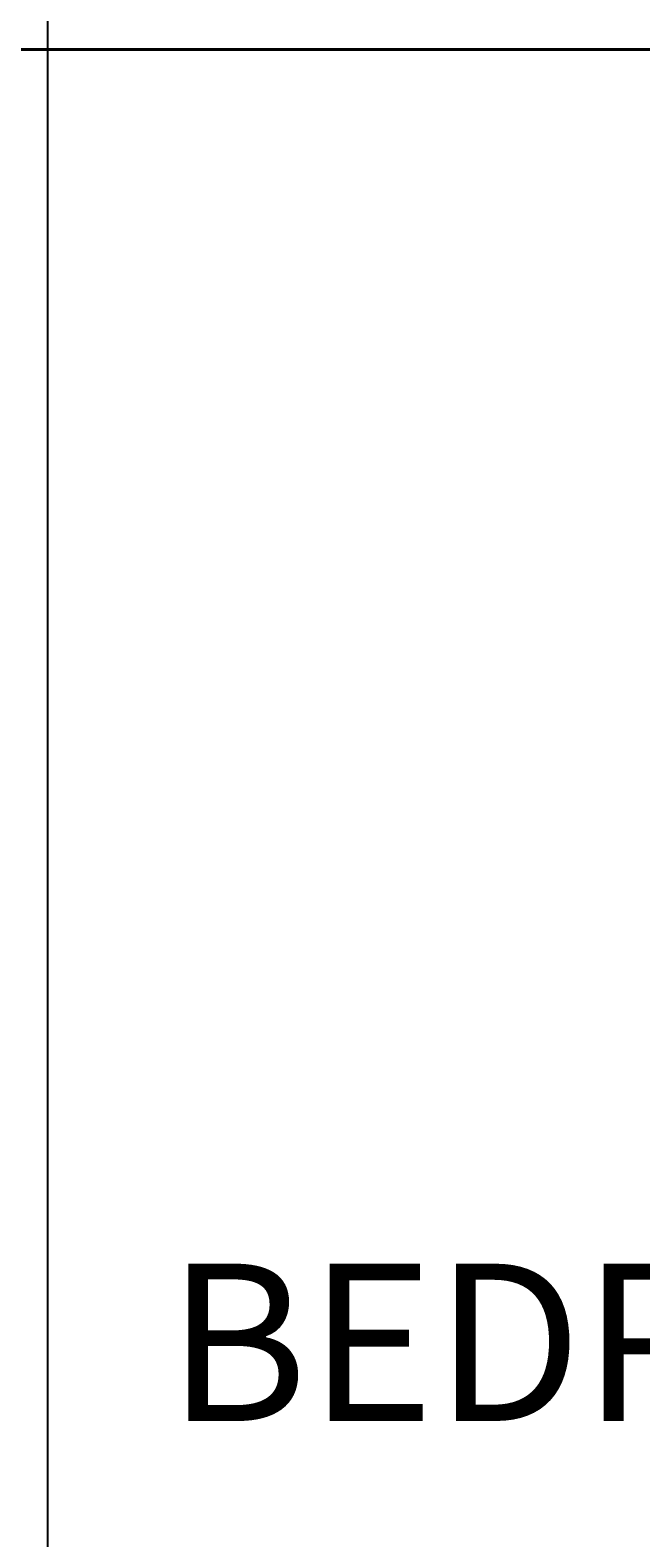
# Model space of a CAD drawing. Units: inches. Extents: x -301 to 715, y -607 to 364.
# Tile 83 of 141: x -123 to -92, y -10 to 67. Entities that reach past the tile are written whole.
import ezdxf

# ---------------------------------------------------------------- set-up
doc = ezdxf.new("R2010")
doc.units = ezdxf.units.IN
doc.header["$MEASUREMENT"] = 0
for name, color, linetype, lineweight in [('A-ANNO-DIMS', 2, 'Continuous', 18), ('A-AREA-IDEN', 220, 'Continuous', 25), ('A-WALL', 3, 'Continuous', 40)]:
    doc.layers.add(name, color=color, linetype=linetype, lineweight=lineweight)
doc.styles.get("Standard").update_dxf_attribs({"font": 'arial.ttf'})
doc.dimstyles.get("Standard").update_dxf_attribs({"dimtxt": 0.18, "dimasz": 0.18, "dimexe": 0.18, "dimexo": 0.0625, "dimgap": 0.09, "dimtad": 0, "dimtih": 1, "dimtoh": 1, "dimdec": 1, "dimzin": 0, "dimdsep": 46, "dimlunit": 4, "dimtxsty": 'Standard', "dimcen": 0.09, "dimclrd": 3, "dimclre": 4, "dimclrt": 6, "dimadec": 0, "dimazin": 0, "dimtfac": 1, "dimtdec": 1, "dimtofl": 0, "dimtmove": 0, "dimatfit": 3, "dimfxl": 1, "dimtfill": 2, "dimtfillclr": 51, "dimtolj": 1, "dimtzin": 0, "dimarcsym": 0})

# ---------------------------------------------------------------- blocks, each defined once
blk = doc.blocks.new('*D151')
at = {"layer": 'A-ANNO-DIMS', "color": 4, "lineweight": -2, "transparency": 16777216}
for p, q in [((-204.603, -223.755), (-204.603, 359.612)), ((-45.603, -214.755), (-45.603, 359.612))]:
    blk.add_line(p, q, dxfattribs=at)
at = {"layer": 'A-ANNO-DIMS', "color": 3, "lineweight": -2, "transparency": 16777216}
for p, q in [((-204.423, 359.432), (-125.494, 359.432)), ((-45.783, 359.432), (-124.713, 359.432))]:
    blk.add_line(p, q, dxfattribs=at)
at = {"layer": 'A-ANNO-DIMS', "color": 3, "transparency": 16777216}
for points in [[(-204.423, 359.462), (-204.423, 359.402), (-204.603, 359.432)], [(-45.783, 359.462), (-45.783, 359.402), (-45.603, 359.432)]]:
    blk.add_solid(points, dxfattribs=at)
at = {"layer": 'Defpoints', "color": 0, "transparency": 16777216}
for p in [(-45.603, 359.432), (-45.603, -214.818), (-204.603, -223.818)]:
    blk.add_point(p, dxfattribs=at)
at = {"layer": 'A-ANNO-DIMS', "color": 6, "transparency": 16777216, "insert": (-125.103, 359.432), "char_height": 0.18, "attachment_point": 5, "bg_fill": 1, "box_fill_scale": 1.25, "bg_fill_color": 51, "bg_fill_transparency": 0}
blk.add_mtext('\\A1;13\'-3"', dxfattribs=at)
blk = doc.blocks.new('*D158')
at = {"layer": 'A-ANNO-DIMS', "color": 4, "lineweight": -2, "transparency": 16777216}
for p, q in [((-122.603, 221.62), (-122.603, -296.865)), ((-50.603, 221.62), (-50.603, -296.865))]:
    blk.add_line(p, q, dxfattribs=at)
at = {"layer": 'A-ANNO-DIMS', "color": 3, "lineweight": -2, "transparency": 16777216}
for p, q in [((-122.423, -296.685), (-86.933, -296.685)), ((-50.783, -296.685), (-86.274, -296.685))]:
    blk.add_line(p, q, dxfattribs=at)
at = {"layer": 'A-ANNO-DIMS', "color": 3, "transparency": 16777216}
for points in [[(-122.423, -296.655), (-122.423, -296.715), (-122.603, -296.685)], [(-50.783, -296.655), (-50.783, -296.715), (-50.603, -296.685)]]:
    blk.add_solid(points, dxfattribs=at)
at = {"layer": 'Defpoints', "color": 0, "transparency": 16777216}
for p in [(-122.603, 221.682), (-50.603, 221.682), (-50.603, -296.685)]:
    blk.add_point(p, dxfattribs=at)
at = {"layer": 'A-ANNO-DIMS', "color": 6, "transparency": 16777216, "insert": (-86.603, -296.685), "char_height": 0.18, "attachment_point": 5, "bg_fill": 1, "box_fill_scale": 1.25, "bg_fill_color": 51, "bg_fill_transparency": 0}
blk.add_mtext('\\A1;6\'-0"', dxfattribs=at)

msp = doc.modelspace()

# ---------------------------------------------------------------- linework, layer by layer
at = {"layer": 'A-WALL'}
msp.add_line((-45.603, 65.682), (-195.603, 65.682), dxfattribs=at)

# ---------------------------------------------------------------- texts
at = {"layer": 'A-AREA-IDEN', "insert": (-116.542, 3.934), "char_height": 8, "attachment_point": 1}
msp.add_mtext_dynamic_manual_height_columns('BEDROOM', width=73.06001, gutter_width=1, heights=[0], dxfattribs=at)

# ---------------------------------------------------------------- dimensions: what is measured, and where the dimension line sits
at = {"layer": 'A-ANNO-DIMS'}
for base, p1, p2, picture, middle in [((-45.603, 359.432), (-204.603, -223.818), (-45.603, -214.818), '*D151', (-125.103, 359.432)), ((-50.603, -296.685), (-122.603, 221.682), (-50.603, 221.682), '*D158', (-86.603, -296.685))]:
    dim = msp.add_linear_dim(base=base, p1=p1, p2=p2, dimstyle='Standard', override={"dimdec": 1, "dimlfac": 1, "dimrnd": 0, "dimzin": 1, "dimdsep": 46, "dimlunit": 4, "dimfrac": 2}, dxfattribs=at)
    dim.commit()
    dim.dimension.update_dxf_attribs({"geometry": picture, "text_midpoint": middle})

doc.saveas('drawing.dxf')
